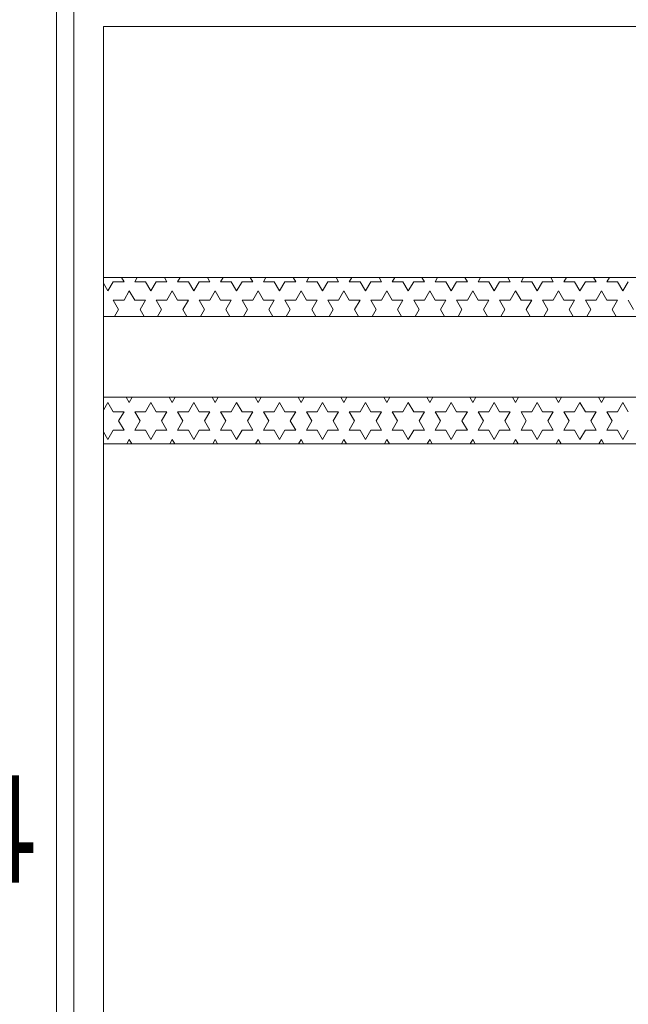
# Model space of a CAD drawing. Units: inches. Extents: x 1291 to 2095, y 532 to 1090.
# Tile 6 of 14: x 1618 to 1640, y 761 to 798. Entities that reach past the tile are written whole.
import ezdxf

# ---------------------------------------------------------------- set-up
doc = ezdxf.new("R2010")
doc.units = ezdxf.units.IN
doc.header["$MEASUREMENT"] = 0
doc.layers.add('A-ANNO-DIMS', color=2, linetype='Continuous', lineweight=18)
doc.layers.add('A-FURN', color=8, linetype='Continuous', lineweight=18)
doc.styles.get("Standard").update_dxf_attribs({"font": 'arial.ttf'})
doc.dimstyles.get("Standard").update_dxf_attribs({"dimtxt": 4, "dimasz": 0.18, "dimexe": 0.18, "dimexo": 0.0625, "dimgap": 0.09, "dimtad": 0, "dimtih": 1, "dimtoh": 1, "dimdec": 0, "dimrnd": 6, "dimzin": 0, "dimdsep": 46, "dimlunit": 3, "dimtxsty": 'Standard', "dimcen": 0.09, "dimadec": 0, "dimazin": 0, "dimtfac": 1, "dimtdec": 0, "dimtofl": 0, "dimtmove": 0, "dimatfit": 3, "dimfxl": 1, "dimtolj": 1, "dimtzin": 0, "dimarcsym": 0})

# ---------------------------------------------------------------- blocks, each defined once
blk = doc.blocks.new('A$C73B76B3A')
for p, q in [((1.35, 0), (1.35, 2)), ((1.33, 1.98), (1.33, 0.02)), ((1.2954, 0.0644), (1.2954, 1.5889)), ((1.2954, 0.5509), (0.0673, 0.5509)), ((0.6839, 0.535), (0.6902, 0.5459)), ((0.6964, 0.535), (0.6902, 0.5459)), ((0.7152, 0.5459), (0.7123, 0.5509)), ((0.7152, 0.5459), (0.7181, 0.5509)), ((0.7339, 0.535), (0.7402, 0.5459)), ((0.7464, 0.535), (0.7402, 0.5459)), ((0.7652, 0.5459), (0.7623, 0.5509)), ((0.7652, 0.5459), (0.7681, 0.5509)), ((0.7839, 0.535), (0.7902, 0.5459)), ((0.7964, 0.535), (0.7902, 0.5459)), ((0.8152, 0.5459), (0.8123, 0.5509)), ((0.8152, 0.5459), (0.8181, 0.5509)), ((0.8339, 0.535), (0.8402, 0.5459)), ((0.8464, 0.535), (0.8402, 0.5459)), ((0.8652, 0.5459), (0.8623, 0.5509)), ((0.8652, 0.5459), (0.8681, 0.5509)), ((0.8839, 0.535), (0.8902, 0.5459)), ((0.8964, 0.535), (0.8902, 0.5459)), ((0.9152, 0.5459), (0.9123, 0.5509)), ((0.9152, 0.5459), (0.9181, 0.5509)), ((0.9339, 0.535), (0.9402, 0.5459)), ((0.9464, 0.535), (0.9402, 0.5459)), ((0.9652, 0.5459), (0.9623, 0.5509)), ((0.9652, 0.5459), (0.9681, 0.5509)), ((0.9839, 0.535), (0.9902, 0.5459)), ((0.9964, 0.535), (0.9902, 0.5459)), ((1.0152, 0.5459), (1.0123, 0.5509)), ((1.0152, 0.5459), (1.0181, 0.5509)), ((1.0339, 0.535), (1.0402, 0.5459)), ((1.0464, 0.535), (1.0402, 0.5459)), ((1.0652, 0.5459), (1.0623, 0.5509)), ((1.0652, 0.5459), (1.0681, 0.5509)), ((1.0839, 0.535), (1.0902, 0.5459)), ((1.0964, 0.535), (1.0902, 0.5459)), ((1.1152, 0.5459), (1.1123, 0.5509)), ((1.1152, 0.5459), (1.1181, 0.5509)), ((1.1339, 0.535), (1.1402, 0.5459)), ((1.1464, 0.535), (1.1402, 0.5459)), ((1.1652, 0.5459), (1.1623, 0.5509)), ((1.1652, 0.5459), (1.1681, 0.5509)), ((1.1839, 0.535), (1.1902, 0.5459)), ((1.1964, 0.535), (1.1902, 0.5459)), ((1.2152, 0.5459), (1.2123, 0.5509)), ((1.2152, 0.5459), (1.2181, 0.5509)), ((1.2339, 0.535), (1.2402, 0.5459)), ((1.2464, 0.535), (1.2402, 0.5459)), ((1.2652, 0.5459), (1.2623, 0.5509)), ((1.2652, 0.5459), (1.2681, 0.5509)), ((1.2839, 0.535), (1.2902, 0.5459)), ((1.2954, 0.5368), (1.2902, 0.5459)), ((0.6964, 0.535), (0.7089, 0.535)), ((0.7027, 0.5242), (0.7089, 0.535)), ((0.7214, 0.535), (0.7339, 0.535)), ((0.7277, 0.5242), (0.7214, 0.535)), ((0.7464, 0.535), (0.7589, 0.535)), ((0.7527, 0.5242), (0.7589, 0.535)), ((0.7714, 0.535), (0.7839, 0.535)), ((0.7777, 0.5242), (0.7714, 0.535)), ((0.7964, 0.535), (0.8089, 0.535)), ((0.8027, 0.5242), (0.8089, 0.535)), ((0.8214, 0.535), (0.8339, 0.535)), ((0.8277, 0.5242), (0.8214, 0.535)), ((0.8464, 0.535), (0.8589, 0.535)), ((0.8527, 0.5242), (0.8589, 0.535)), ((0.8714, 0.535), (0.8839, 0.535)), ((0.8777, 0.5242), (0.8714, 0.535)), ((0.8964, 0.535), (0.9089, 0.535)), ((0.9027, 0.5242), (0.9089, 0.535)), ((0.9214, 0.535), (0.9339, 0.535)), ((0.9277, 0.5242), (0.9214, 0.535)), ((0.9464, 0.535), (0.9589, 0.535)), ((0.9527, 0.5242), (0.9589, 0.535)), ((0.9714, 0.535), (0.9839, 0.535)), ((0.9777, 0.5242), (0.9714, 0.535)), ((0.9964, 0.535), (1.0089, 0.535)), ((1.0027, 0.5242), (1.0089, 0.535)), ((1.0214, 0.535), (1.0339, 0.535)), ((1.0277, 0.5242), (1.0214, 0.535)), ((1.0464, 0.535), (1.0589, 0.535)), ((1.0527, 0.5242), (1.0589, 0.535)), ((1.0714, 0.535), (1.0839, 0.535)), ((1.0777, 0.5242), (1.0714, 0.535)), ((1.0964, 0.535), (1.1089, 0.535)), ((1.1027, 0.5242), (1.1089, 0.535)), ((1.1214, 0.535), (1.1339, 0.535)), ((1.1277, 0.5242), (1.1214, 0.535)), ((1.1464, 0.535), (1.1589, 0.535)), ((1.1527, 0.5242), (1.1589, 0.535)), ((1.1714, 0.535), (1.1839, 0.535)), ((1.1777, 0.5242), (1.1714, 0.535)), ((1.1964, 0.535), (1.2089, 0.535)), ((1.2027, 0.5242), (1.2089, 0.535)), ((1.2214, 0.535), (1.2339, 0.535)), ((1.2277, 0.5242), (1.2214, 0.535)), ((1.2464, 0.535), (1.2589, 0.535)), ((1.2527, 0.5242), (1.2589, 0.535)), ((1.2714, 0.535), (1.2839, 0.535)), ((1.2777, 0.5242), (1.2714, 0.535)), ((0.7089, 0.5134), (0.7027, 0.5242)), ((0.7214, 0.5134), (0.7277, 0.5242)), ((0.7589, 0.5134), (0.7527, 0.5242)), ((0.7714, 0.5134), (0.7777, 0.5242)), ((0.8089, 0.5134), (0.8027, 0.5242)), ((0.8214, 0.5134), (0.8277, 0.5242)), ((0.8589, 0.5134), (0.8527, 0.5242)), ((0.8714, 0.5134), (0.8777, 0.5242)), ((0.9089, 0.5134), (0.9027, 0.5242)), ((0.9214, 0.5134), (0.9277, 0.5242)), ((0.9589, 0.5134), (0.9527, 0.5242)), ((0.9714, 0.5134), (0.9777, 0.5242)), ((1.0089, 0.5134), (1.0027, 0.5242)), ((1.0214, 0.5134), (1.0277, 0.5242)), ((1.0589, 0.5134), (1.0527, 0.5242)), ((1.0714, 0.5134), (1.0777, 0.5242)), ((1.1089, 0.5134), (1.1027, 0.5242)), ((1.1214, 0.5134), (1.1277, 0.5242)), ((1.1589, 0.5134), (1.1527, 0.5242)), ((1.1714, 0.5134), (1.1777, 0.5242)), ((1.2089, 0.5134), (1.2027, 0.5242)), ((1.2214, 0.5134), (1.2277, 0.5242)), ((1.2589, 0.5134), (1.2527, 0.5242)), ((1.2714, 0.5134), (1.2777, 0.5242)), ((0.6902, 0.5026), (0.6839, 0.5134)), ((0.6902, 0.5026), (0.6964, 0.5134)), ((0.6964, 0.5134), (0.7089, 0.5134)), ((0.7214, 0.5134), (0.7339, 0.5134)), ((0.7402, 0.5026), (0.7339, 0.5134)), ((0.7402, 0.5026), (0.7464, 0.5134)), ((0.7464, 0.5134), (0.7589, 0.5134)), ((0.7714, 0.5134), (0.7839, 0.5134)), ((0.7902, 0.5026), (0.7839, 0.5134)), ((0.7902, 0.5026), (0.7964, 0.5134)), ((0.7964, 0.5134), (0.8089, 0.5134)), ((0.8214, 0.5134), (0.8339, 0.5134)), ((0.8402, 0.5026), (0.8339, 0.5134)), ((0.8402, 0.5026), (0.8464, 0.5134)), ((0.8464, 0.5134), (0.8589, 0.5134)), ((0.8714, 0.5134), (0.8839, 0.5134)), ((0.8902, 0.5026), (0.8839, 0.5134)), ((0.8902, 0.5026), (0.8964, 0.5134)), ((0.8964, 0.5134), (0.9089, 0.5134)), ((0.9214, 0.5134), (0.9339, 0.5134)), ((0.9402, 0.5026), (0.9339, 0.5134)), ((0.9402, 0.5026), (0.9464, 0.5134)), ((0.9464, 0.5134), (0.9589, 0.5134)), ((0.9714, 0.5134), (0.9839, 0.5134)), ((0.9902, 0.5026), (0.9839, 0.5134)), ((0.9902, 0.5026), (0.9964, 0.5134)), ((0.9964, 0.5134), (1.0089, 0.5134)), ((1.0214, 0.5134), (1.0339, 0.5134)), ((1.0402, 0.5026), (1.0339, 0.5134)), ((1.0402, 0.5026), (1.0464, 0.5134)), ((1.0464, 0.5134), (1.0589, 0.5134)), ((1.0714, 0.5134), (1.0839, 0.5134)), ((1.0902, 0.5026), (1.0839, 0.5134)), ((1.0902, 0.5026), (1.0964, 0.5134)), ((1.0964, 0.5134), (1.1089, 0.5134)), ((1.1214, 0.5134), (1.1339, 0.5134)), ((1.1402, 0.5026), (1.1339, 0.5134)), ((1.1402, 0.5026), (1.1464, 0.5134)), ((1.1464, 0.5134), (1.1589, 0.5134)), ((1.1714, 0.5134), (1.1839, 0.5134)), ((1.1902, 0.5026), (1.1839, 0.5134)), ((1.1902, 0.5026), (1.1964, 0.5134)), ((1.1964, 0.5134), (1.2089, 0.5134)), ((1.2214, 0.5134), (1.2339, 0.5134)), ((1.2402, 0.5026), (1.2339, 0.5134)), ((1.2402, 0.5026), (1.2464, 0.5134)), ((1.2464, 0.5134), (1.2589, 0.5134)), ((1.2714, 0.5134), (1.2839, 0.5134)), ((1.2902, 0.5026), (1.2839, 0.5134)), ((1.2902, 0.5026), (1.2954, 0.5116)), ((1.2954, 0.4965), (0.0673, 0.4965)), ((0.7117, 0.4965), (0.7152, 0.5026)), ((0.7187, 0.4965), (0.7152, 0.5026)), ((0.7617, 0.4965), (0.7652, 0.5026)), ((0.7687, 0.4965), (0.7652, 0.5026)), ((0.8117, 0.4965), (0.8152, 0.5026)), ((0.8187, 0.4965), (0.8152, 0.5026)), ((0.8617, 0.4965), (0.8652, 0.5026)), ((0.8687, 0.4965), (0.8652, 0.5026)), ((0.9117, 0.4965), (0.9152, 0.5026)), ((0.9187, 0.4965), (0.9152, 0.5026)), ((0.9617, 0.4965), (0.9652, 0.5026)), ((0.9687, 0.4965), (0.9652, 0.5026)), ((1.0117, 0.4965), (1.0152, 0.5026)), ((1.0187, 0.4965), (1.0152, 0.5026)), ((1.0617, 0.4965), (1.0652, 0.5026)), ((1.0687, 0.4965), (1.0652, 0.5026)), ((1.1117, 0.4965), (1.1152, 0.5026)), ((1.1187, 0.4965), (1.1152, 0.5026)), ((1.1617, 0.4965), (1.1652, 0.5026)), ((1.1687, 0.4965), (1.1652, 0.5026)), ((1.2117, 0.4965), (1.2152, 0.5026)), ((1.2187, 0.4965), (1.2152, 0.5026)), ((1.2617, 0.4965), (1.2652, 0.5026)), ((1.2687, 0.4965), (1.2652, 0.5026)), ((1.2954, 0.4023), (0.0673, 0.4023)), ((0.7027, 0.3943), (0.6981, 0.4023)), ((0.7277, 0.3943), (0.7323, 0.4023)), ((0.7527, 0.3943), (0.7481, 0.4023)), ((0.7777, 0.3943), (0.7823, 0.4023)), ((0.8027, 0.3943), (0.7981, 0.4023)), ((0.8277, 0.3943), (0.8323, 0.4023)), ((0.8527, 0.3943), (0.8481, 0.4023)), ((0.8777, 0.3943), (0.8823, 0.4023)), ((0.9027, 0.3943), (0.8981, 0.4023)), ((0.9277, 0.3943), (0.9323, 0.4023)), ((0.9527, 0.3943), (0.9481, 0.4023)), ((0.9777, 0.3943), (0.9823, 0.4023)), ((1.0027, 0.3943), (0.9981, 0.4023)), ((1.0277, 0.3943), (1.0323, 0.4023)), ((1.0527, 0.3943), (1.0481, 0.4023)), ((1.0777, 0.3943), (1.0823, 0.4023)), ((1.1027, 0.3943), (1.0981, 0.4023)), ((1.1277, 0.3943), (1.1323, 0.4023)), ((1.1527, 0.3943), (1.1481, 0.4023)), ((1.1777, 0.3943), (1.1823, 0.4023)), ((1.2027, 0.3943), (1.1981, 0.4023)), ((1.2277, 0.3943), (1.2323, 0.4023)), ((1.2527, 0.3943), (1.2481, 0.4023)), ((1.2777, 0.3943), (1.2823, 0.4023)), ((0.6839, 0.3835), (0.6777, 0.3943)), ((0.6964, 0.3835), (0.7027, 0.3943)), ((0.7339, 0.3835), (0.7277, 0.3943)), ((0.7464, 0.3835), (0.7527, 0.3943)), ((0.7839, 0.3835), (0.7777, 0.3943)), ((0.7964, 0.3835), (0.8027, 0.3943)), ((0.8339, 0.3835), (0.8277, 0.3943)), ((0.8464, 0.3835), (0.8527, 0.3943)), ((0.8839, 0.3835), (0.8777, 0.3943)), ((0.8964, 0.3835), (0.9027, 0.3943)), ((0.9339, 0.3835), (0.9277, 0.3943)), ((0.9464, 0.3835), (0.9527, 0.3943)), ((0.9839, 0.3835), (0.9777, 0.3943)), ((0.9964, 0.3835), (1.0027, 0.3943)), ((1.0339, 0.3835), (1.0277, 0.3943)), ((1.0464, 0.3835), (1.0527, 0.3943)), ((1.0839, 0.3835), (1.0777, 0.3943)), ((1.0964, 0.3835), (1.1027, 0.3943)), ((1.1339, 0.3835), (1.1277, 0.3943)), ((1.1464, 0.3835), (1.1527, 0.3943)), ((1.1839, 0.3835), (1.1777, 0.3943)), ((1.1964, 0.3835), (1.2027, 0.3943)), ((1.2339, 0.3835), (1.2277, 0.3943)), ((1.2464, 0.3835), (1.2527, 0.3943)), ((1.2839, 0.3835), (1.2777, 0.3943)), ((0.6964, 0.3835), (0.7089, 0.3835)), ((0.7152, 0.3726), (0.7089, 0.3835)), ((0.7152, 0.3726), (0.7214, 0.3835)), ((0.7214, 0.3835), (0.7339, 0.3835)), ((0.7464, 0.3835), (0.7589, 0.3835)), ((0.7652, 0.3726), (0.7589, 0.3835)), ((0.7652, 0.3726), (0.7714, 0.3835)), ((0.7714, 0.3835), (0.7839, 0.3835)), ((0.7964, 0.3835), (0.8089, 0.3835)), ((0.8152, 0.3726), (0.8089, 0.3835)), ((0.8152, 0.3726), (0.8214, 0.3835)), ((0.8214, 0.3835), (0.8339, 0.3835)), ((0.8464, 0.3835), (0.8589, 0.3835)), ((0.8652, 0.3726), (0.8589, 0.3835)), ((0.8652, 0.3726), (0.8714, 0.3835)), ((0.8714, 0.3835), (0.8839, 0.3835)), ((0.8964, 0.3835), (0.9089, 0.3835)), ((0.9152, 0.3726), (0.9089, 0.3835)), ((0.9152, 0.3726), (0.9214, 0.3835)), ((0.9214, 0.3835), (0.9339, 0.3835)), ((0.9464, 0.3835), (0.9589, 0.3835)), ((0.9652, 0.3726), (0.9589, 0.3835)), ((0.9652, 0.3726), (0.9714, 0.3835)), ((0.9714, 0.3835), (0.9839, 0.3835)), ((0.9964, 0.3835), (1.0089, 0.3835)), ((1.0152, 0.3726), (1.0089, 0.3835)), ((1.0152, 0.3726), (1.0214, 0.3835)), ((1.0214, 0.3835), (1.0339, 0.3835)), ((1.0464, 0.3835), (1.0589, 0.3835)), ((1.0652, 0.3726), (1.0589, 0.3835)), ((1.0652, 0.3726), (1.0714, 0.3835)), ((1.0714, 0.3835), (1.0839, 0.3835)), ((1.0964, 0.3835), (1.1089, 0.3835)), ((1.1152, 0.3726), (1.1089, 0.3835)), ((1.1152, 0.3726), (1.1214, 0.3835)), ((1.1214, 0.3835), (1.1339, 0.3835)), ((1.1464, 0.3835), (1.1589, 0.3835)), ((1.1652, 0.3726), (1.1589, 0.3835)), ((1.1652, 0.3726), (1.1714, 0.3835)), ((1.1714, 0.3835), (1.1839, 0.3835)), ((1.1964, 0.3835), (1.2089, 0.3835)), ((1.2152, 0.3726), (1.2089, 0.3835)), ((1.2152, 0.3726), (1.2214, 0.3835)), ((1.2214, 0.3835), (1.2339, 0.3835)), ((1.2464, 0.3835), (1.2589, 0.3835)), ((1.2652, 0.3726), (1.2589, 0.3835)), ((1.2652, 0.3726), (1.2714, 0.3835)), ((1.2714, 0.3835), (1.2839, 0.3835)), ((0.6839, 0.3618), (0.6902, 0.3726)), ((0.6964, 0.3618), (0.6902, 0.3726)), ((0.7339, 0.3618), (0.7402, 0.3726)), ((0.7464, 0.3618), (0.7402, 0.3726)), ((0.7839, 0.3618), (0.7902, 0.3726)), ((0.7964, 0.3618), (0.7902, 0.3726)), ((0.8339, 0.3618), (0.8402, 0.3726)), ((0.8464, 0.3618), (0.8402, 0.3726)), ((0.8839, 0.3618), (0.8902, 0.3726)), ((0.8964, 0.3618), (0.8902, 0.3726)), ((0.9339, 0.3618), (0.9402, 0.3726)), ((0.9464, 0.3618), (0.9402, 0.3726)), ((0.9839, 0.3618), (0.9902, 0.3726)), ((0.9964, 0.3618), (0.9902, 0.3726)), ((1.0339, 0.3618), (1.0402, 0.3726)), ((1.0464, 0.3618), (1.0402, 0.3726)), ((1.0839, 0.3618), (1.0902, 0.3726)), ((1.0964, 0.3618), (1.0902, 0.3726)), ((1.1339, 0.3618), (1.1402, 0.3726)), ((1.1464, 0.3618), (1.1402, 0.3726)), ((1.1839, 0.3618), (1.1902, 0.3726)), ((1.1964, 0.3618), (1.1902, 0.3726)), ((1.2339, 0.3618), (1.2402, 0.3726)), ((1.2464, 0.3618), (1.2402, 0.3726)), ((1.2839, 0.3618), (1.2902, 0.3726)), ((1.2954, 0.3636), (1.2902, 0.3726)), ((1.2954, 0.3568), (0.0673, 0.3568)), ((0.6964, 0.3618), (0.7089, 0.3618)), ((0.706, 0.3568), (0.7089, 0.3618)), ((0.7214, 0.3618), (0.7339, 0.3618)), ((0.7243, 0.3568), (0.7214, 0.3618)), ((0.7464, 0.3618), (0.7589, 0.3618)), ((0.756, 0.3568), (0.7589, 0.3618)), ((0.7714, 0.3618), (0.7839, 0.3618)), ((0.7743, 0.3568), (0.7714, 0.3618)), ((0.7964, 0.3618), (0.8089, 0.3618)), ((0.806, 0.3568), (0.8089, 0.3618)), ((0.8214, 0.3618), (0.8339, 0.3618)), ((0.8243, 0.3568), (0.8214, 0.3618)), ((0.8464, 0.3618), (0.8589, 0.3618)), ((0.856, 0.3568), (0.8589, 0.3618)), ((0.8714, 0.3618), (0.8839, 0.3618)), ((0.8743, 0.3568), (0.8714, 0.3618)), ((0.8964, 0.3618), (0.9089, 0.3618)), ((0.906, 0.3568), (0.9089, 0.3618)), ((0.9214, 0.3618), (0.9339, 0.3618)), ((0.9243, 0.3568), (0.9214, 0.3618)), ((0.9464, 0.3618), (0.9589, 0.3618)), ((0.956, 0.3568), (0.9589, 0.3618)), ((0.9714, 0.3618), (0.9839, 0.3618)), ((0.9743, 0.3568), (0.9714, 0.3618)), ((0.9964, 0.3618), (1.0089, 0.3618)), ((1.006, 0.3568), (1.0089, 0.3618)), ((1.0214, 0.3618), (1.0339, 0.3618)), ((1.0243, 0.3568), (1.0214, 0.3618)), ((1.0464, 0.3618), (1.0589, 0.3618)), ((1.056, 0.3568), (1.0589, 0.3618)), ((1.0714, 0.3618), (1.0839, 0.3618)), ((1.0743, 0.3568), (1.0714, 0.3618)), ((1.0964, 0.3618), (1.1089, 0.3618)), ((1.106, 0.3568), (1.1089, 0.3618)), ((1.1214, 0.3618), (1.1339, 0.3618)), ((1.1243, 0.3568), (1.1214, 0.3618)), ((1.1464, 0.3618), (1.1589, 0.3618)), ((1.156, 0.3568), (1.1589, 0.3618)), ((1.1714, 0.3618), (1.1839, 0.3618)), ((1.1743, 0.3568), (1.1714, 0.3618)), ((1.1964, 0.3618), (1.2089, 0.3618)), ((1.206, 0.3568), (1.2089, 0.3618)), ((1.2214, 0.3618), (1.2339, 0.3618)), ((1.2243, 0.3568), (1.2214, 0.3618)), ((1.2464, 0.3618), (1.2589, 0.3618)), ((1.256, 0.3568), (1.2589, 0.3618)), ((1.2714, 0.3618), (1.2839, 0.3618)), ((1.2743, 0.3568), (1.2714, 0.3618)), ((0.0673, 0.0644), (1.2954, 0.0644))]:
    blk.add_line(p, q)
blk = doc.blocks.new('*D30')
at = {"layer": 'A-ANNO-DIMS', "color": 0, "lineweight": -2, "transparency": 16777216}
for p, q in [((1618.87, 799.814), (1609.145, 799.814)), ((1609.325, 799.634), (1609.325, 769.922)), ((1609.325, 735.946), (1609.325, 765.658)), ((1618.87, 735.766), (1609.145, 735.766))]:
    blk.add_line(p, q, dxfattribs=at)
at = {"layer": 'A-ANNO-DIMS', "color": 0, "transparency": 16777216}
for points in [[(1609.295, 799.634), (1609.355, 799.634), (1609.325, 799.814)], [(1609.295, 735.946), (1609.355, 735.946), (1609.325, 735.766)]]:
    blk.add_solid(points, dxfattribs=at)
at = {"layer": 'Defpoints', "color": 0, "transparency": 16777216}
for p in [(1618.932, 799.814), (1609.325, 735.766), (1618.932, 735.766)]:
    blk.add_point(p, dxfattribs=at)
at = {"layer": 'A-ANNO-DIMS', "color": 0, "transparency": 16777216, "insert": (1609.325, 767.79), "char_height": 4, "attachment_point": 5}
blk.add_mtext('\\A1;BED 64', dxfattribs=at)
blk = doc.blocks.new('*D46')
at = {"layer": 'A-ANNO-DIMS', "color": 0, "lineweight": -2, "transparency": 16777216}
for p, q in [((1600.27, 579.843), (1600.27, 1087.16)), ((1685.584, 579.843), (1685.584, 1087.16)), ((1600.45, 1086.98), (1636.471, 1086.98)), ((1685.404, 1086.98), (1649.383, 1086.98))]:
    blk.add_line(p, q, dxfattribs=at)
at = {"layer": 'A-ANNO-DIMS', "color": 0, "transparency": 16777216}
for points in [[(1600.45, 1087.01), (1600.45, 1086.95), (1600.27, 1086.98)], [(1685.404, 1087.01), (1685.404, 1086.95), (1685.584, 1086.98)]]:
    blk.add_solid(points, dxfattribs=at)
at = {"layer": 'Defpoints', "color": 0, "transparency": 16777216}
for p in [(1685.584, 1086.98), (1600.27, 579.78), (1685.584, 579.78)]:
    blk.add_point(p, dxfattribs=at)
at = {"layer": 'A-ANNO-DIMS', "color": 0, "transparency": 16777216, "insert": (1642.927, 1086.98), "char_height": 4, "attachment_point": 5}
blk.add_mtext('\\A1;85.31', dxfattribs=at)
blk = doc.blocks.new('*D49')
at = {"layer": 'A-ANNO-DIMS', "color": 0, "lineweight": -2, "transparency": 16777216}
for p, q in [((1694.074, 852.718), (1694.074, 534.4)), ((1586.074, 816.718), (1586.074, 534.4)), ((1586.254, 534.58), (1635.749, 534.58)), ((1693.894, 534.58), (1644.398, 534.58))]:
    blk.add_line(p, q, dxfattribs=at)
at = {"layer": 'A-ANNO-DIMS', "color": 0, "transparency": 16777216}
for points in [[(1586.254, 534.61), (1586.254, 534.55), (1586.074, 534.58)], [(1693.894, 534.61), (1693.894, 534.55), (1694.074, 534.58)]]:
    blk.add_solid(points, dxfattribs=at)
at = {"layer": 'Defpoints', "color": 0, "transparency": 16777216}
for p in [(1694.074, 852.78), (1586.074, 816.78), (1694.074, 534.58)]:
    blk.add_point(p, dxfattribs=at)
at = {"layer": 'A-ANNO-DIMS', "color": 0, "transparency": 16777216, "insert": (1640.074, 534.58), "char_height": 4, "attachment_point": 5}
blk.add_mtext('\\A1;108', dxfattribs=at)
blk = doc.blocks.new('*D51')
at = {"layer": 'A-ANNO-DIMS', "color": 0, "lineweight": -2, "transparency": 16777216}
for p, q in [((1820.011, 852.78), (1297.694, 852.78)), ((1297.874, 852.6), (1297.874, 794.913)), ((1297.874, 732.96), (1297.874, 790.648)), ((1811.011, 732.78), (1297.694, 732.78))]:
    blk.add_line(p, q, dxfattribs=at)
at = {"layer": 'A-ANNO-DIMS', "color": 0, "transparency": 16777216}
for points in [[(1297.844, 852.6), (1297.904, 852.6), (1297.874, 852.78)], [(1297.844, 732.96), (1297.904, 732.96), (1297.874, 732.78)]]:
    blk.add_solid(points, dxfattribs=at)
at = {"layer": 'Defpoints', "color": 0, "transparency": 16777216}
for p in [(1297.874, 852.78), (1820.074, 852.78), (1811.074, 732.78)]:
    blk.add_point(p, dxfattribs=at)
at = {"layer": 'A-ANNO-DIMS', "color": 0, "transparency": 16777216, "insert": (1297.874, 792.78), "char_height": 4, "attachment_point": 5}
blk.add_mtext('\\A1;120', dxfattribs=at)

msp = doc.modelspace()

# ---------------------------------------------------------------- block references
at = {"layer": 'A-FURN', "xscale": 32.02427574694497, "yscale": 32.02427574694497, "zscale": 32.02427574694497, "rotation": 180}
msp.add_blockref('A$C73B76B3A', (1662.1648, 799.8143), dxfattribs=at)

# ---------------------------------------------------------------- dimensions: what is measured, and where the dimension line sits
at = {"layer": 'A-ANNO-DIMS'}
for base, p1, p2, override, picture, middle in [((1685.5842, 1086.9804), (1600.2697, 579.7804), (1685.5842, 579.7804), {"dimdec": 2, "dimlfac": 1, "dimrnd": 0, "dimzin": 0, "dimdsep": 46, "dimlunit": 2}, '*D46', (1642.927, 1086.9804)), ((1694.0735, 534.5804), (1586.0735, 816.7804), (1694.0735, 852.7804), {"dimdec": 0, "dimlfac": 1, "dimrnd": 0, "dimzin": 0, "dimdsep": 46, "dimlunit": 2}, '*D49', (1640.0735, 534.5804))]:
    dim = msp.add_linear_dim(base=base, p1=p1, p2=p2, dimstyle='Standard', override=override, dxfattribs=at)
    dim.commit()
    dim.dimension.update_dxf_attribs({"geometry": picture, "text_midpoint": middle})
dim = msp.add_linear_dim(base=(1297.8735, 852.7804), p1=(1811.0735, 732.7804), p2=(1820.0735, 852.7804), angle=90, dimstyle='Standard', override={"dimdec": 0, "dimlfac": 1, "dimrnd": 0, "dimzin": 0, "dimdsep": 46, "dimlunit": 2}, dxfattribs=at)
dim.commit()
dim.dimension.update_dxf_attribs({"geometry": '*D51', "text_midpoint": (1297.8735, 792.7804)})
dim = msp.add_linear_dim(base=(1609.3247, 735.7658), p1=(1618.932, 799.8143), p2=(1618.932, 735.7658), angle=270, text='BED <>', dimstyle='Standard', override={"dimdec": 0, "dimlfac": 1, "dimrnd": 0, "dimzin": 0, "dimdsep": 46, "dimlunit": 2}, dxfattribs=at)
dim.commit()
dim.dimension.update_dxf_attribs({"geometry": '*D30', "text_midpoint": (1609.3247, 767.79)})

doc.saveas('drawing.dxf')
